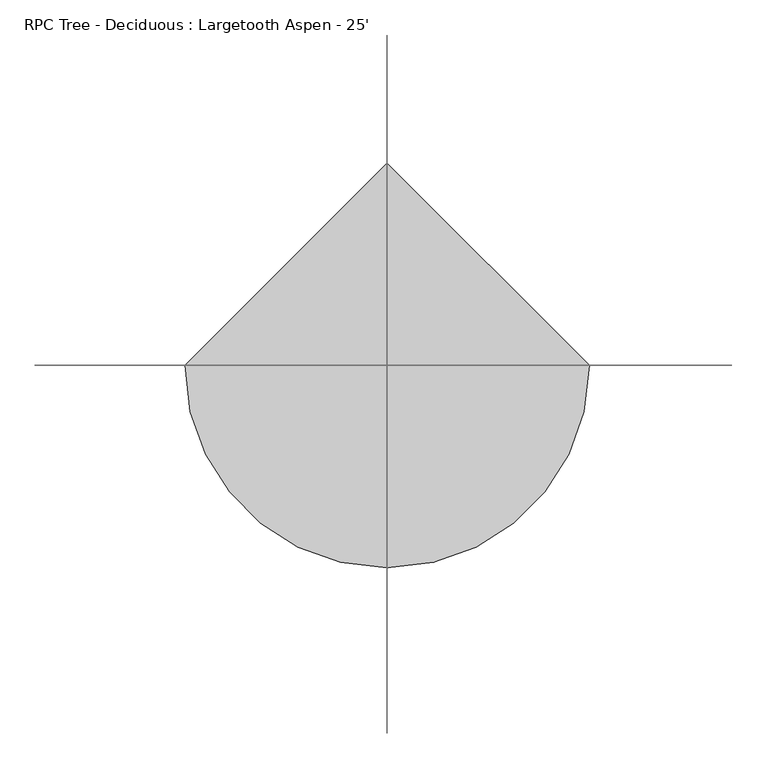
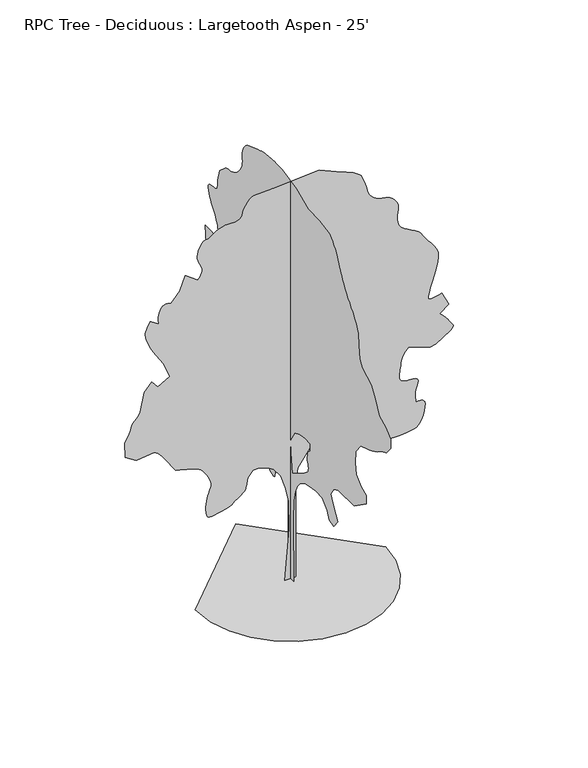
"""IFC4 building model written with IfcOpenShell, lengths in millimetres: geographic element geometry, RPC Tree - Deciduous : Largetooth Aspen - 25'."""

from ifc_helpers import new_model, si_unit, origin, place, context, project, spatial, triangles, source, transform, mapped, element, save


def rpc_tree_deciduous_largetooth_aspen_25_f6cd7aa4(model_context):
    return source(origin(), model_context, "Body", "Tessellation", [
        triangles([(93.1061447, 0.000407, 0.0055275), (-104.1894253, 0.000407, 0.0055275), (-22.9504001, 0.0003503, 951.6658939), (-34.5559031, 0.0003185, 1485.5251682), (-92.5836657, 0.0003019, 1764.061219), (-173.8237105, 0.0002874, 2007.7790462), (-301.4849952, 0.000277, 2181.8628971), (-405.9347789, 0.0002735, 2239.8916225), (-568.4133425, 0.0002701, 2297.9204933), (-684.470866, 0.0002701, 2297.9204933), (-765.710166, 0.000277, 2181.8628971), (-800.5284622, 0.000286, 2030.9895481), (-803.4037228, 0.000287, 2013.4305908), (-808.6158319, 0.0002881, 1994.9546837), (-818.4938627, 0.0002893, 1974.6550507), (-835.3797506, 0.0002907, 1951.6121258), (-861.6001705, 0.0002923, 1924.9168076), (-899.4969126, 0.0002942, 1893.6518555), (-951.4017385, 0.0002963, 1856.9058426), (-1000.9367964, 0.0002984, 1821.7851665), (-1035.041328, 0.0003, 1794.7824543), (-1061.0280413, 0.0003013, 1774.0764507), (-1086.2019407, 0.0003023, 1757.8357269), (-1117.8706472, 0.0003031, 1744.2340862), (-1163.3467958, 0.0003038, 1731.4425705), (-1229.9353912, 0.0003046, 1717.6377445), (-1303.2575146, 0.0003056, 1701.9735844), (-1364.6008633, 0.0003064, 1687.5234489), (-1414.7786144, 0.000307, 1678.356712), (-1454.6032185, 0.000307, 1678.5242889), (-1484.8875618, 0.0003062, 1692.0929375), (-1506.439444, 0.0003043, 1723.119096), (-1520.076693, 0.0003012, 1775.66647), (-1526.0305447, 0.0002975, 1838.229221), (-1525.0830734, 0.000294, 1896.7304466), (-1518.8575813, 0.0002907, 1951.3759483), (-1508.9769344, 0.0002877, 2002.3662952), (-1497.0669056, 0.0002848, 2049.9049633), (-1484.7505062, 0.0002822, 2094.1948471), (-1473.6532185, 0.0002797, 2135.4418934), (-1462.0149754, 0.0002776, 2171.5098953), (-1448.7511047, 0.0002758, 2202.2997311), (-1436.5031605, 0.000274, 2231.0600395), (-1427.9079002, 0.0002723, 2261.0397503), (-1425.6065872, 0.0002702, 2295.4845955), (-1432.2385952, 0.0002677, 2337.6435047), (-1450.4427166, 0.0002645, 2390.7649715), (-1477.2752357, 0.0002611, 2448.2171333), (-1507.353923, 0.000258, 2500.7976448), (-1539.6676483, 0.0002552, 2547.8968048), (-1573.1981598, 0.0002527, 2588.9178474), (-1606.9320019, 0.0002507, 2623.2079056), (-1639.8528122, 0.0002491, 2650.2080017), (-1670.950042, 0.0002479, 2669.3088707), (-1706.2051575, 0.000247, 2684.2184258), (-1751.2088058, 0.0002461, 2699.1535606), (-1804.330418, 0.0002453, 2714.0634064), (-1863.9491627, 0.0002444, 2728.9985413), (-1928.439703, 0.0002435, 2743.908387), (-1996.1788822, 0.0002426, 2758.8182327), (-2065.5412182, 0.0002417, 2773.7533676), (-2262.8354256, 0.0002244, 3063.8972855), (-2307.8392193, 0.0002208, 3124.7302002), (-2344.3134464, 0.0002181, 3169.7390808), (-2373.6809853, 0.0002162, 3201.539756), (-2397.3664581, 0.0002149, 3222.7742157), (-2416.7872204, 0.0002141, 3236.1091576), (-2433.3683304, 0.0002137, 3244.1609917), (-2448.5269981, 0.0002133, 3249.5711266), (-2773.4740242, 0.0002154, 3214.7732506), (-2970.7811668, 0.0002078, 3342.4334816), (-2982.3888885, 0.0001919, 3609.3616653), (-2960.1129227, 0.0001895, 3649.1127274), (-2938.5738304, 0.0001872, 3688.6606041), (-2918.4317459, 0.0001848, 3727.8273994), (-2900.4229614, 0.0001825, 3766.3590591), (-2885.2846413, 0.0001803, 3804.0779778), (-2873.6769196, 0.0001781, 3840.78097), (-2866.3363792, 0.000176, 3876.2901398), (-2854.8809738, 0.000174, 3909.843615), (-2833.1131165, 0.0001721, 3941.5934212), (-2804.8174599, 0.0001702, 3972.5051971), (-2773.8803947, 0.0001684, 4003.6457382), (-2744.1877304, 0.0001665, 4035.9798111), (-2719.5499901, 0.0001644, 4070.5745018), (-2703.8526924, 0.0001621, 4108.3951584), (-2634.2060715, 0.0001414, 4456.5779755), (-2494.950618, 0.0001324, 4607.4283607), (-2390.4982727, 0.00014, 4479.7681297), (-2169.9909473, 0.0001331, 4595.8459282), (-2286.0485435, 0.0001158, 4885.9645569), (-2471.7375, 9.85e-05, 5176.1084747), (-2494.0692764, 9.6e-05, 5217.3577011), (-2519.6494011, 9.3e-05, 5268.7673538), (-2546.0425575, 8.96e-05, 5326.2475662), (-2570.8076157, 8.6e-05, 5385.7596313), (-2591.5086777, 8.26e-05, 5443.2398438), (-2605.7325188, 7.95e-05, 5494.6494965), (-2611.0159172, 7.71e-05, 5535.8993042), (-2608.2980598, 7.5e-05, 5570.3669678), (-2600.7287544, 7.3e-05, 5604.2503647), (-2589.0701637, 7.1e-05, 5637.6006546), (-2574.1858978, 6.9e-05, 5670.544574), (-2556.863118, 6.71e-05, 5703.2088593), (-2537.9197975, 6.52e-05, 5735.6446701), (-2518.1611198, 6.32e-05, 5768.0037415), (-2367.2877708, 6.95e-05, 5663.5595352), (-2372.0934368, 6.75e-05, 5695.9697662), (-2375.8831764, 6.56e-05, 5728.8881058), (-2377.6407726, 6.35e-05, 5762.8226624), (-2376.3555313, 6.14e-05, 5798.2809631), (-2371.00891, 5.92e-05, 5835.7711166), (-2360.5873077, 5.68e-05, 5875.8018127), (-2344.077269, 5.42e-05, 5918.8799973), (-2322.4899239, 5.2e-05, 5956.5480469), (-2297.8569798, 5.05e-05, 5981.4145523), (-2270.6865452, 4.97e-05, 5995.6131042), (-2241.4867287, 4.93e-05, 6001.3028732), (-2210.7630226, 4.94e-05, 6000.5918701), (-2179.0257156, 4.97e-05, 5995.6131042), (-2146.7804455, 5.01e-05, 5988.501329), (-1995.9070965, 3.97e-05, 6162.5924469), (-1891.4573673, 2.45e-05, 6417.9129089), (-1670.950042, 3.42e-05, 6255.4298035), (-1648.8215961, 3.24e-05, 6285.3250717), (-1628.2145691, 3.06e-05, 6315.3988174), (-1610.6529957, 2.88e-05, 6345.8789337), (-1597.6609108, 2.69e-05, 6376.9683151), (-1590.7597332, 2.5e-05, 6408.8960175), (-1591.4684109, 2.31e-05, 6441.814357), (-1601.3160656, 2.1e-05, 6475.9523895), (-1617.3536041, 1.89e-05, 6510.877002), (-1634.407069, 1.68e-05, 6546.3864624), (-1650.6477928, 1.46e-05, 6583.140033), (-1664.2495789, 1.23e-05, 6621.7225616), (-1673.3859398, 9.9e-06, 6662.7183151), (-1676.2282082, 7.3e-06, 6706.761557), (-1670.950042, 4.4e-06, 6754.488295), (-1658.2957272, 1.5e-06, 6803.2306686), (-1640.7672913, -1.2e-06, 6848.9505524), (-1619.1798008, -3.6e-06, 6889.9968842), (-1594.3462875, -5.7e-06, 6924.7441818), (-1567.0742603, -7.3e-06, 6951.5663818), (-1538.1767509, -8.4e-06, 6968.8641632), (-1508.471442, -8.7e-06, 6974.9853012), (-1475.2102455, -9.2e-06, 6983.3417679), (-1435.6574272, -1.05e-05, 7004.9067307), (-1390.6206413, -1.23e-05, 7034.3706299), (-1340.9153904, -1.42e-05, 7066.4762283), (-1287.3545609, -1.59e-05, 7095.9401276), (-1230.7481323, -1.72e-05, 7117.504509), (-1171.9065931, -1.77e-05, 7125.861557), (-1111.9499331, -1.77e-05, 7125.5313446), (-1053.2124573, -1.77e-05, 7125.9882935), (-998.3307781, -1.79e-05, 7129.5188919), (-949.9463768, -1.85e-05, 7138.307309), (-910.695793, -1.94e-05, 7154.6138718), (-883.2205805, -2.1e-05, 7180.6744904), (-870.1599678, -2.32e-05, 7218.6983322), (-859.1973375, -2.62e-05, 7267.6691803), (-837.8816328, -2.94e-05, 7321.8984283), (-808.6488241, -3.27e-05, 7376.76194), (-773.9321205, -3.57e-05, 7427.5367477), (-736.1725794, -3.82e-05, 7469.5992966), (-697.8033371, -3.99e-05, 7498.2504547), (-661.2603642, -4.05e-05, 7508.8422501), (-324.6980224, -4.19e-05, 7532.0576935), (510.9103117, -4.54e-05, 7590.0965927), (928.7119898, -3.43e-05, 7404.3974625), (997.9725878, -3.27e-05, 7376.9148376), (1065.003162, -3.1e-05, 7348.7462082), (1127.5632969, -2.92e-05, 7319.1294113), (1183.4279829, -2.73e-05, 7287.4051849), (1230.3570225, -2.53e-05, 7252.8102036), (1266.1201012, -2.3e-05, 7214.6852051), (1288.4873405, -2.05e-05, 7172.2924438), (1303.3743679, -1.8e-05, 7130.6618454), (1318.0580647, -1.58e-05, 7093.7303787), (1332.3378616, -1.37e-05, 7059.0086609), (1346.0081028, -1.16e-05, 7024.0834671), (1358.8656029, -9.4e-06, 6986.5171555), (1370.7070312, -6.9e-06, 6943.8959198), (1381.3319641, -3.9e-06, 6893.7565384), (1397.2017803, -8e-07, 6841.9149353), (1423.0183731, 2e-06, 6795.9665771), (1455.9391834, 4.3e-06, 6756.1137772), (1493.1248497, 6.3e-06, 6722.5350128), (1531.7301968, 7.9e-06, 6695.4843384), (1568.915863, 9.2e-06, 6675.1134888), (1601.8392895, 1e-05, 6661.6259399), (1632.2912098, 1.04e-05, 6653.548526), (1663.5535458, 1.08e-05, 6648.1133926), (1695.0215378, 1.1e-05, 6643.6683151), (1726.0831593, 1.13e-05, 6638.6389709), (1756.1288544, 1.18e-05, 6631.3492996), (1784.5513927, 1.24e-05, 6620.2238159), (1810.7387478, 1.34e-05, 6603.6126205), (1836.0828403, 1.48e-05, 6581.0320221), (1861.4244621, 1.64e-05, 6553.8028702), (1885.3461124, 1.82e-05, 6522.9169647), (1906.4256397, 2.02e-05, 6489.3887787), (1923.2429272, 2.23e-05, 6454.2351105), (1934.3756779, 2.45e-05, 6418.4721771), (1938.4015949, 2.66e-05, 6383.0900345), (1934.8836411, 2.9e-05, 6341.7640686), (1927.3043072, 3.21e-05, 6289.6434128), (1920.1313438, 3.57e-05, 6230.2325043), (1917.8301762, 3.94e-05, 6166.9613663), (1924.8685547, 4.32e-05, 6103.2838577), (1945.7117592, 4.69e-05, 6042.6538376), (1984.8250694, 5.01e-05, 5988.501329), (2039.569693, 5.28e-05, 5943.162236), (2101.6243355, 5.51e-05, 5904.3256531), (2166.9277622, 5.72e-05, 5868.5371399), (2231.4183025, 5.94e-05, 5832.3166763), (2291.0370472, 6.18e-05, 5792.2609818), (2341.7227615, 6.46e-05, 5744.890036), (2379.4162457, 6.81e-05, 5686.7749786), (2417.9887459, 7.19e-05, 5621.9795151), (2469.1466698, 7.58e-05, 5556.3713104), (2525.585376, 7.98e-05, 5489.1376236), (2580.0024033, 8.4e-05, 5419.4657135), (2625.0618622, 8.83e-05, 5346.5422577), (2653.4845459, 9.29e-05, 5269.5800949), (2657.9549126, 9.78e-05, 5187.7164871), (2641.5719009, 0.0001035, 5093.1519104), (2615.0543335, 0.00011, 4983.9574127), (2582.4409172, 0.0001169, 4868.2862755), (2547.7697777, 0.0001237, 4754.2147499), (2515.1639191, 0.0001299, 4649.8972801), (2488.6361778, 0.000135, 4563.4609863), (2472.2607239, 0.0001386, 4502.9835732), (2471.4479828, 0.0001408, 4466.6872421), (2487.0816216, 0.000142, 4445.6050987), (2516.4161682, 0.0001425, 4437.2230522), (2556.710511, 0.0001424, 4438.9758522), (2605.2247009, 0.0001419, 4448.3482452), (2659.2248932, 0.000141, 4462.8008514), (2715.9685226, 0.00014, 4479.7681297), (2843.6287537, 0.0001552, 4224.4476677), (2681.1706467, 0.0001628, 4096.7874367), (2705.9862831, 0.0001642, 4074.3338654), (2730.6243141, 0.0001655, 4051.3466057), (2754.8559746, 0.000167, 4027.3692902), (2778.4777885, 0.0001685, 4001.8420692), (2801.2868614, 0.0001701, 3974.3085754), (2823.0802986, 0.0001719, 3944.2351204), (2843.6287537, 0.0001739, 3911.1135956), (2865.6250854, 0.0001758, 3878.8553902), (2888.8408195, 0.0001775, 3850.6614716), (2908.8050079, 0.000179, 3824.931356), (2921.0478653, 0.0001805, 3799.9886925), (2921.1240234, 0.0001821, 3774.2329971), (2904.5378265, 0.0001837, 3746.0643677), (2866.8441971, 0.0001857, 3713.8064529), (2611.523735, 0.000196, 3539.7150444), (2507.076622, 0.0001967, 3528.1073227), (2124.0931675, 0.0001891, 3655.7675537), (2096.88727, 0.0001908, 3628.2340599), (2070.5983223, 0.0001925, 3599.5829018), (2046.1355713, 0.0001943, 3568.6964149), (2024.4110252, 0.0001964, 3534.4319366), (2006.3439594, 0.0001987, 3495.74767), (1992.8439114, 0.0002013, 3451.4500832), (1984.8250694, 0.0002043, 3400.4470917), (1979.2422707, 0.0002073, 3350.9425552), (1972.8464401, 0.0002097, 3309.9723816), (1966.2475697, 0.0002118, 3274.6916862), (1960.0550697, 0.0002138, 3242.2305862), (1954.8784962, 0.0002157, 3209.7947754), (1951.3250793, 0.0002178, 3174.4887909), (1950.0068459, 0.0002203, 3133.5186172), (1959.0060059, 0.0002226, 3094.8599304), (1982.2191238, 0.0002242, 3067.1485405), (2013.9564308, 0.0002253, 3048.55578), (2048.5358608, 0.000226, 3037.3035599), (2080.2731678, 0.0002263, 3031.5123436), (2103.4861404, 0.0002265, 3029.3787529), (2112.4854458, 0.0002265, 3029.0738297), (2125.1752235, 0.0002264, 3029.9630196), (2157.148708, 0.0002264, 3030.4202591), (2199.274625, 0.0002266, 3027.2451622), (2242.4164684, 0.0002272, 3017.1614754), (2277.4354065, 0.0002284, 2996.942942), (2295.2001652, 0.0002304, 2963.2880196), (2286.5717674, 0.0002334, 2913.021611), (2265.7615551, 0.0002368, 2855.3635025), (2252.261507, 0.0002401, 2801.3633102), (2244.8497501, 0.0002431, 2750.4108971), (2242.3122597, 0.000246, 2701.871418), (2243.429924, 0.0002488, 2655.1864769), (2246.9833408, 0.0002515, 2609.7203568), (2251.7533985, 0.0002541, 2564.8385033), (2291.2047695, 0.0002539, 2569.2835808), (2328.629084, 0.0002538, 2570.4774033), (2361.9894024, 0.0002541, 2565.1434265), (2389.2612843, 0.000255, 2550.1065536), (2408.4128769, 0.0002567, 2522.0472198), (2417.4120369, 0.0002593, 2477.7574814), (2414.2319984, 0.0002631, 2413.9754734), (2401.476091, 0.0002675, 2341.0953289), (2383.2389774, 0.0002716, 2272.8811787), (2359.7236977, 0.0002752, 2211.166777), (2331.1309662, 0.0002784, 2157.7735245), (2297.6690552, 0.000281, 2114.5300884), (2259.536063, 0.0002829, 2083.2677525), (2216.9377911, 0.0002839, 2065.807917), (2176.9759861, 0.0002844, 2057.1795193), (2143.1075592, 0.0002848, 2050.7838341), (2110.049548, 0.0002851, 2046.0136311), (2072.5261116, 0.0002853, 2042.257029), (2025.2567585, 0.0002855, 2038.9092682), (1962.9659386, 0.0002857, 2035.3558514), (1880.3728695, 0.000286, 2030.9895481), (1790.6068371, 0.0002859, 2032.4449825), (1709.3674644, 0.0002851, 2045.4726757), (1635.2326, 0.0002838, 2068.1420769), (1566.7847431, 0.0002819, 2098.5255421), (1502.5989807, 0.0002798, 2134.6977528), (1441.2554867, 0.0002774, 2174.7255421), (1381.3319641, 0.0002749, 2216.6811207), (1126.0062698, 0.0002604, 2460.3989479), (859.0779408, 0.0002535, 2576.4465157), (545.7260645, 0.0002548, 2553.2563614), (394.8527518, 0.0002618, 2437.1885914), (290.4029863, 0.0002708, 2286.3152424), (127.9229058, 0.0002846, 2054.2026661), (93.1061447, 0.0003019, 1764.061219), (93.1061447, 0.0003392, 1137.3575392), (-0.0023708, 90.8437737, 1.11e-05), (-0.0023708, -94.8460457, 0.0), (-0.0023708, -83.2405405, 1160.5629541), (-0.0023708, -94.8460457, 1531.9435558), (-0.0023708, -141.2688208, 1729.2379086), (-0.0023708, -210.9025882, 1880.1112576), (-0.0023708, -303.7481383, 1996.1687084), (-0.0023708, -443.0162001, 2077.4080811), (-0.0023708, -559.0712165, 2100.6185829), (-0.0023708, -791.1838291, 2147.0420574), (-0.0023708, -988.4806526, 2135.4368065), (-0.0023708, -1139.3539289, 1984.5634575), (-0.0023708, -1208.987978, 1845.2955048), (-0.0023708, -1336.648209, 1798.8718849), (-0.0023708, -1475.9163071, 1972.9557358), (-0.0023708, -1325.0429581, 2205.0707829), (-0.0023708, -1255.4089817, 2367.5493828), (-0.0023708, -1336.648209, 2506.8150101), (-0.0023708, -1487.521558, 2576.4465157), (-0.0023708, -1974.9572124, 2576.4465157), (-0.0023708, -2357.9431377, 2843.3746994), (-0.0023708, -2357.9431377, 3005.8583862), (-0.0023708, -2195.4645378, 3075.479718), (-0.0023708, -2044.5913342, 3214.7476707), (-0.0023708, -2009.7755814, 3412.0548134), (-0.0023708, -2032.9860832, 3644.159832), (-0.0023708, -2183.8592869, 3841.466684), (-0.0023708, -2450.787616, 3934.3037498), (-0.0023708, -2495.4866318, 3951.778846), (-0.0023708, -2539.7763702, 3969.5332855), (-0.0023708, -2583.2536583, 3987.8975716), (-0.0023708, -2625.5191017, 4007.2016258), (-0.0023708, -2666.159063, 4027.6995026), (-0.0023708, -2704.7671715, 4049.7211235), (-0.0023708, -2740.9367661, 4073.5717026), (-0.0023708, -2775.734642, 4097.0920692), (-0.0023708, -2810.5580978, 4118.1742126), (-0.0023708, -2845.381263, 4137.223922), (-0.0023708, -2880.2047188, 4154.6484398), (-0.0023708, -2915.0025948, 4170.8535553), (-0.0023708, -2949.8260506, 4186.2459297), (-0.0023708, -2984.6495064, 4201.2319336), (-0.0023708, -3112.3097374, 4363.7156204), (-0.0023708, -3112.3097374, 4526.1993073), (-0.0023708, -2961.4337723, 4665.46726), (-0.0023708, -2764.1522095, 4769.9120476), (-0.0023708, -2636.4666893, 5013.6247879), (-0.0023708, -2508.8189575, 5199.3239182), (-0.0023708, -2230.2829067, 5350.1995926), (-0.0023708, -2149.0435341, 5477.860405), (-0.0023708, -2125.8305614, 5733.180867), (-0.0023708, -2102.6200596, 5942.0698608), (-0.0023708, -2077.7179459, 5994.1655182), (-0.0023708, -2052.6126469, 6045.3211166), (-0.0023708, -2027.0983612, 6094.647757), (-0.0023708, -2000.9769905, 6141.2315414), (-0.0023708, -1974.0453495, 6184.1824081), (-0.0023708, -1946.0953114, 6222.5364624), (-0.0023708, -1916.9309578, 6255.4298035), (-0.0023708, -1880.7588924, 6294.3169647), (-0.0023708, -1835.0490372, 6347.6061539), (-0.0023708, -1784.4624447, 6409.8360764), (-0.0023708, -1733.6777538, 6475.4948593), (-0.0023708, -1687.355872, 6539.1473694), (-0.0023708, -1650.170351, 6595.2811523), (-0.0023708, -1626.7896561, 6638.4104965), (-0.0023708, -1609.9062389, 6674.6559586), (-0.0023708, -1589.7741829, 6713.7465958), (-0.0023708, -1567.4070889, 6755.6568283), (-0.0023708, -1543.8256794, 6800.4366531), (-0.0023708, -1520.0386139, 6848.0360733), (-0.0023708, -1497.0642895, 6898.4806686), (-0.0023708, -1475.9163071, 6951.7698578), (-0.0023708, -1452.6372047, 7005.1352051), (-0.0023708, -1423.2671951, 7056.0623291), (-0.0023708, -1388.8223499, 7104.957019), (-0.0023708, -1350.3185955, 7152.2262268), (-0.0023708, -1308.7667713, 7198.2763229), (-0.0023708, -1265.188036, 7243.513678), (-0.0023708, -1220.5932289, 7288.3446625), (-0.0023708, -895.6335583, 7346.3585632), (-0.0023708, -547.4659656, 7357.9659943), (-0.0023708, -176.0855819, 7520.4496811), (-0.0023708, 264.9268161, 7613.2870377), (-0.0023708, 324.5456334, 7615.7252609), (-0.0023708, 383.7580439, 7617.8588516), (-0.0023708, 442.1602203, 7619.3825958), (-0.0023708, 499.3406327, 7619.9924423), (-0.0023708, 554.9005408, 7619.3825958), (-0.0023708, 608.4284509, 7617.2490051), (-0.0023708, 659.5204994, 7613.2870377), (-0.0023708, 708.649114, 7608.2065338), (-0.0023708, 756.9649876, 7602.5423447), (-0.0023708, 805.0801466, 7595.6340454), (-0.0023708, 853.6016762, 7586.8962067), (-0.0023708, 903.136734, 7575.7457245), (-0.0023708, 954.2948032, 7561.5215927), (-0.0023708, 1007.6881285, 7543.6657059), (-0.0023708, 1344.2529774, 7427.6129059), (-0.0023708, 1373.9607571, 7402.5429245), (-0.0023708, 1402.8557957, 7376.228833), (-0.0023708, 1430.1278229, 7347.5015167), (-0.0023708, 1454.9613361, 7315.141864), (-0.0023708, 1476.5488266, 7277.8801849), (-0.0023708, 1494.0772625, 7234.5479462), (-0.0023708, 1506.7315773, 7183.8748764), (-0.0023708, 1511.0952644, 7135.4627151), (-0.0023708, 1507.5418476, 7096.3970764), (-0.0023708, 1500.9454479, 7061.7770966), (-0.0023708, 1496.1727741, 7026.7507462), (-0.0023708, 1498.1031796, 6986.4659958), (-0.0023708, 1511.6032276, 6935.996402), (-0.0023708, 1541.5473301, 6870.5405136), (-0.0023708, 1582.5555828, 6804.0434097), (-0.0023708, 1625.189463, 6752.1768082), (-0.0023708, 1668.2270977, 6712.4769058), (-0.0023708, 1710.4546074, 6682.5298965), (-0.0023708, 1750.6525898, 6659.8987198), (-0.0023708, 1787.5994625, 6642.1439896), (-0.0023708, 1820.0833809, 6626.8024841), (-0.0023708, 1849.9258907, 6615.6775818), (-0.0023708, 1879.7682552, 6610.2418671), (-0.0023708, 1909.6107651, 6607.6257477), (-0.0023708, 1939.4557457, 6605.0346268), (-0.0023708, 1969.2981102, 6599.5739136), (-0.0023708, 1999.14062, 6588.4484299), (-0.0023708, 2028.9829845, 6568.7891647), (-0.0023708, 2203.0693062, 6417.9129089), (-0.0023708, 2272.7008118, 6197.4159027), (-0.0023708, 2270.435107, 6162.7197647), (-0.0023708, 2269.4877811, 6128.8613663), (-0.0023708, 2271.179393, 6096.6034515), (-0.0023708, 2276.8307922, 6066.8093399), (-0.0023708, 2287.7578869, 6040.2411942), (-0.0023708, 2305.2864681, 6017.7367538), (-0.0023708, 2330.7295372, 6000.1087601), (-0.0023708, 2366.121999, 5990.0250732), (-0.0023708, 2409.2282341, 5986.2404205), (-0.0023708, 2454.9736977, 5983.6754608), (-0.0023708, 2498.2855888, 5977.2491089), (-0.0023708, 2534.0819504, 5961.8820236), (-0.0023708, 2557.2947777, 5932.4942825), (-0.0023708, 2562.8319397, 5884.0565414), (-0.0023708, 2554.1452606, 5827.7448624), (-0.0023708, 2538.7528862, 5777.5287415), (-0.0023708, 2517.7724808, 5732.3931244), (-0.0023708, 2492.3292664, 5691.3217941), (-0.0023708, 2463.5359657, 5653.2979523), (-0.0023708, 2432.5073364, 5617.3059631), (-0.0023708, 2400.3636589, 5582.3046112), (-0.0023708, 2375.59613, 5540.0391678), (-0.0023708, 2351.4381569, 5497.9004608), (-0.0023708, 2328.49697, 5455.9402313), (-0.0023708, 2307.3844505, 5414.284053), (-0.0023708, 2288.7053581, 5373.0342453), (-0.0023708, 2273.0741901, 5332.2931274), (-0.0023708, 2261.0955608, 5292.1606934), (-0.0023708, 2254.8700687, 5254.4164856), (-0.0023708, 2255.3450397, 5220.3046143), (-0.0023708, 2261.4003387, 5189.2402313), (-0.0023708, 2271.9235336, 5160.614653), (-0.0023708, 2285.7971054, 5133.8174515), (-0.0023708, 2301.9032444, 5108.2399429), (-0.0023708, 2319.1244316, 5083.2716995), (-0.0023708, 2469.9977806, 5106.4871429), (-0.0023708, 2655.6942947, 5106.4871429), (-0.0023708, 2632.4788513, 4769.9120476), (-0.0023708, 2423.5741608, 4410.1467979), (-0.0023708, 2416.0988903, 4367.9066437), (-0.0023708, 2408.5195564, 4325.9967018), (-0.0023708, 2400.7370373, 4284.6710266), (-0.0023708, 2392.6495949, 4244.2848289), (-0.0023708, 2384.1559273, 4205.0927444), (-0.0023708, 2375.1567673, 4167.4246948), (-0.0023708, 2365.5479061, 4131.6106018), (-0.0023708, 2351.1663712, 4092.901046), (-0.0023708, 2330.0869892, 4047.8924561), (-0.0023708, 2305.5556377, 3998.8448685), (-0.0023708, 2280.8237171, 3947.9433243), (-0.0023708, 2259.134634, 3897.4737305), (-0.0023708, 2243.7397888, 3849.620256), (-0.0023708, 2237.885059, 3806.6435188), (-0.0023708, 2242.6221245, 3768.5435188), (-0.0023708, 2255.8859951, 3733.4915886), (-0.0023708, 2276.2542286, 3700.9796196), (-0.0023708, 2302.3069988, 3670.4995033), (-0.0023708, 2332.6244797, 3641.5181328), (-0.0023708, 2365.7840836, 3613.5782684), (-0.0023708, 2400.3636589, 3586.1462219), (-0.0023708, 2713.7079048, 3655.7675537), (-0.0023708, 2731.0053955, 3606.110701), (-0.0023708, 2747.5915924, 3556.834639), (-0.0023708, 2762.7552017, 3508.3968979), (-0.0023708, 2775.7599312, 3461.1529793), (-0.0023708, 2785.945356, 3415.5345428), (-0.0023708, 2792.5748932, 3371.9482498), (-0.0023708, 2794.9625381, 3330.8257599), (-0.0023708, 2781.5002785, 3291.6333847), (-0.0023708, 2746.9055878, 3253.2540413), (-0.0023708, 2699.9410126, 3215.103463), (-0.0023708, 2649.3188118, 3176.5209343), (-0.0023708, 2603.7768242, 3136.9477684), (-0.0023708, 2572.0523071, 3095.7235405), (-0.0023708, 2562.8319397, 3052.2895638), (-0.0023708, 2571.1886971, 3010.557518), (-0.0023708, 2585.6413033, 2974.3117653), (-0.0023708, 2605.1738319, 2942.6631157), (-0.0023708, 2628.7450676, 2914.6470932), (-0.0023708, 2655.3896622, 2889.3742172), (-0.0023708, 2684.0408203, 2865.9044289), (-0.0023708, 2713.7079048, 2843.3746994), (-0.0023708, 2783.3545258, 2611.2696808), (-0.0023708, 2716.5272095, 2608.9584846), (-0.0023708, 2651.6302986, 2607.7899513), (-0.0023708, 2590.5941986, 2608.8314575), (-0.0023708, 2535.3339088, 2613.225666), (-0.0023708, 2487.7955315, 2622.0902412), (-0.0023708, 2449.8987167, 2636.5428474), (-0.0023708, 2423.5741608, 2657.7008583), (-0.0023708, 2398.2655312, 2683.9137932), (-0.0023708, 2363.2136009, 2712.5649513), (-0.0023708, 2320.0387653, 2743.2479622), (-0.0023708, 2270.3665066, 2775.5823257), (-0.0023708, 2215.8225975, 2809.1102211), (-0.0023708, 2158.0326656, 2843.4508575), (-0.0023708, 2098.6169609, 2878.1981552), (-0.0023708, 2096.1482162, 2840.8347382), (-0.0023708, 2093.7783028, 2803.1919777), (-0.0023708, 2091.6141907, 2764.9143723), (-0.0023708, 2089.7523857, 2725.7219971), (-0.0023708, 2088.2969513, 2685.3360901), (-0.0023708, 2087.3496254, 2643.4008591), (-0.0023708, 2087.01171, 2599.6619591), (-0.0023708, 2085.4216908, 2554.0943916), (-0.0023708, 2079.9734768, 2509.3195084), (-0.0023708, 2069.6534672, 2469.0222588), (-0.0023708, 2053.4457355, 2436.8431183), (-0.0023708, 2030.3368263, 2416.4418926), (-0.0023708, 1999.3108131, 2411.4660336), (-0.0023708, 1959.3490082, 2425.5756374), (-0.0023708, 1914.2462379, 2451.7986008), (-0.0023708, 1868.5363827, 2480.4573166), (-0.0023708, 1822.3160934, 2511.1455597), (-0.0023708, 1775.6894337, 2543.4517273), (-0.0023708, 1728.7603214, 2576.9799133), (-0.0023708, 1681.6281693, 2611.3461296), (-0.0023708, 1634.3918083, 2646.0931366), (-0.0023708, 1355.8582283, 2727.3221901), (-0.0023708, 1077.3221775, 2634.4854149), (-0.0023708, 903.2383266, 2425.5756374), (-0.0023708, 925.671623, 2395.8678577), (-0.0023708, 948.4096247, 2366.9728191), (-0.0023708, 971.754784, 2339.7009373), (-0.0023708, 996.0142771, 2314.8672787), (-0.0023708, 1021.4930271, 2293.2799335), (-0.0023708, 1048.4931959, 2275.7513523), (-0.0023708, 1077.3221775, 2263.0970375), (-0.0023708, 1104.7973173, 2250.7806381), (-0.0023708, 1128.0078192, 2234.2021442), (-0.0023708, 1147.667375, 2214.0700882), (-0.0023708, 1164.4821917, 2191.0957638), (-0.0023708, 1179.1684319, 2165.9904648), (-0.0023708, 1192.4323025, 2139.4627235), (-0.0023708, 1204.984952, 2112.2238338), (-0.0023708, 1172.5694887, 2104.7129551), (-0.0023708, 1139.6486057, 2096.8974438), (-0.0023708, 1105.7091803, 2088.4722313), (-0.0023708, 1070.2508068, 2079.1326851), (-0.0023708, 1032.7604353, 2068.576498), (-0.0023708, 992.7325733, 2056.4962761), (-0.0023708, 949.6593304, 2042.5897121), (-0.0023708, 906.5885582, 2025.6403107), (-0.0023708, 866.5607689, 2005.0332836), (-0.0023708, 829.0703974, 1981.383419), (-0.0023708, 793.6094805, 1955.2951859), (-0.0023708, 759.6725985, 1927.3806107), (-0.0023708, 726.7517155, 1898.2467785), (-0.0023708, 694.3362522, 1868.5060066), (-0.0023708, 694.3362522, 1706.0274067), (-0.0023708, 652.3120005, 1679.1287579), (-0.0023708, 611.8117109, 1654.968314), (-0.0023708, 574.3543679, 1636.2916924), (-0.0023708, 541.4665134, 1625.8370979), (-0.0023708, 514.6695299, 1626.3450611), (-0.0023708, 495.4849088, 1640.556403), (-0.0023708, 485.4341414, 1671.2116539), (-0.0023708, 480.5294263, 1705.9588062), (-0.0023708, 476.0285382, 1733.1976959), (-0.0023708, 472.3404639, 1756.7815762), (-0.0023708, 469.8715739, 1780.5661709), (-0.0023708, 469.025768, 1808.4147617), (-0.0023708, 470.2094167, 1844.1778404), (-0.0023708, 473.8288905, 1891.7165085), (-0.0023708, 476.7727515, 1943.7229271), (-0.0023708, 476.0615667, 1990.8550793), (-0.0023708, 472.3074354, 2033.9283222), (-0.0023708, 466.1149355, 2073.7529263), (-0.0023708, 458.0961662, 2111.1417778), (-0.0023708, 448.8581763, 2146.9074726), (-0.0023708, 439.0131741, 2181.8578102), (-0.0023708, 241.7168229, 2193.4630611), (-0.0023708, 137.2665396, 1996.1687084), (-0.0023708, 79.2382684, 1659.6039322), (-0.0023708, 79.2382684, 1230.1970032), (-0.0023708, 79.2382684, 591.8879997), (-0.0022508, -48.4240337, 2030.9844612), (-0.0022508, -2.0012081, 2402.3651356), (-0.0022508, 9.6043397, 2622.8776932), (-0.0022508, -129.6633155, 2843.3746994), (-0.0022508, -280.5376365, 2913.021611), (-0.0022508, -454.621451, 2936.2117653), (-0.0022508, -617.0999783, 2936.2117653), (-0.0022508, -617.0999783, 2796.9691017), (-0.0022508, -535.8607146, 2727.3221901), (-0.0022508, -512.6502128, 2564.8385033), (-0.0022508, -522.5282799, 2554.7295273), (-0.0022508, -532.0024836, 2543.6043343), (-0.0022508, -540.6638735, 2530.4344986), (-0.0022508, -548.1085862, 2514.226767), (-0.0022508, -553.9277441, 2493.9573647), (-0.0022508, -557.717411, 2468.6158882), (-0.0022508, -559.0712165, 2437.1808884), (-0.0022508, -555.6879564, 2404.7324329), (-0.0022508, -546.2137527, 2376.5486881), (-0.0022508, -531.6646408, 2351.915744), (-0.0022508, -513.0540762, 2330.1250683), (-0.0022508, -491.4006014, 2310.4679832), (-0.0022508, -467.7151285, 2292.2308697), (-0.0022508, -443.0162001, 2274.7022884), (-1711.8591728, 0.0, 0.0031267), (-1666.6040863, -392.2441901, 0.0031033), (-1537.7144245, -752.4590126, 0.0030819), (-1335.5154293, -1070.3218781, 0.0030629), (-1070.3218781, -1335.5154293, 0.0030471), (-752.4590126, -1537.7144245, 0.0030351), (-392.2441901, -1666.6040863, 0.0030274), (7.5e-05, -1711.8591728, 0.0030247), (392.2441901, -1666.6040863, 0.0030274), (752.4590126, -1537.7144245, 0.0030351), (1070.3218781, -1335.5154293, 0.0030471), (1335.5154293, -1070.3218781, 0.0030629), (1537.7144245, -752.4590126, 0.0030819), (1666.6040863, -392.2441901, 0.0031033), (1711.8591728, 0.0001497, 0.0031267), (-0.0002251, 1711.8591728, 0.0032287)], [[122, 123, 124], [87, 88, 89], [1, 2, 3], [329, 1, 3], [329, 3, 4], [328, 329, 4], [328, 4, 5], [105, 106, 107], [327, 328, 5], [327, 5, 6], [104, 105, 107], [238, 239, 240], [238, 240, 241], [237, 238, 241], [236, 237, 241], [103, 104, 107], [86, 87, 89], [235, 236, 241], [102, 103, 107], [101, 102, 107], [100, 101, 107], [99, 100, 107], [98, 99, 107], [97, 98, 107], [96, 97, 107], [327, 6, 7], [326, 327, 7], [95, 96, 107], [70, 71, 72], [69, 70, 72], [69, 72, 73], [69, 73, 74], [69, 74, 75], [69, 75, 76], [69, 76, 77], [69, 77, 78], [94, 95, 107], [234, 235, 241], [93, 94, 107], [69, 78, 79], [69, 79, 80], [69, 80, 81], [69, 81, 82], [69, 82, 83], [69, 83, 84], [69, 84, 85], [68, 69, 85], [325, 326, 7], [325, 7, 8], [67, 68, 85], [92, 93, 107], [91, 92, 107], [60, 61, 62], [67, 85, 86], [67, 86, 89], [67, 89, 90], [66, 67, 90], [65, 66, 90], [64, 65, 90], [63, 64, 90], [62, 63, 90], [60, 62, 90], [59, 60, 90], [58, 59, 90], [57, 58, 90], [56, 57, 90], [55, 56, 90], [54, 55, 90], [53, 54, 90], [284, 285, 286], [283, 284, 286], [282, 283, 286], [282, 286, 287], [281, 282, 287], [280, 281, 287], [279, 280, 287], [279, 287, 288], [278, 279, 288], [277, 278, 288], [277, 288, 289], [276, 277, 289], [275, 276, 289], [275, 289, 290], [52, 53, 90], [325, 8, 9], [121, 122, 124], [275, 290, 291], [30, 31, 32], [29, 30, 32], [29, 32, 33], [28, 29, 33], [28, 33, 34], [27, 28, 34], [27, 34, 35], [27, 35, 36], [26, 27, 36], [26, 36, 37], [26, 37, 38], [25, 26, 38], [25, 38, 39], [24, 25, 39], [23, 24, 39], [22, 23, 39], [21, 22, 39], [20, 21, 39], [20, 39, 40], [20, 40, 41], [20, 41, 42], [19, 20, 42], [19, 42, 43], [18, 19, 43], [18, 43, 44], [17, 18, 44], [16, 17, 44], [15, 16, 44], [14, 15, 44], [13, 14, 44], [12, 13, 44], [11, 12, 44], [11, 44, 45], [11, 45, 46], [10, 11, 46], [10, 46, 47], [10, 47, 48], [10, 48, 49], [10, 49, 50], [10, 50, 51], [252, 253, 254], [251, 252, 254], [251, 254, 255], [250, 251, 255], [249, 250, 255], [249, 255, 256], [248, 249, 256], [247, 248, 256], [246, 247, 256], [245, 246, 256], [245, 256, 257], [245, 257, 258], [244, 245, 258], [243, 244, 258], [242, 243, 258], [241, 242, 258], [234, 241, 258], [233, 234, 258], [274, 275, 291], [324, 325, 9], [51, 52, 90], [10, 51, 90], [9, 10, 90], [324, 9, 90], [323, 324, 90], [323, 90, 91], [323, 91, 107], [323, 107, 108], [323, 108, 109], [323, 109, 110], [323, 110, 111], [323, 111, 112], [323, 112, 113], [323, 113, 114], [323, 114, 115], [323, 115, 116], [323, 116, 117], [323, 117, 118], [323, 118, 119], [323, 119, 120], [323, 120, 121], [323, 121, 124], [323, 124, 125], [323, 125, 126], [323, 126, 127], [323, 127, 128], [323, 128, 129], [322, 323, 129], [322, 129, 130], [167, 168, 169], [274, 291, 292], [296, 297, 298], [296, 298, 299], [295, 296, 299], [294, 295, 299], [294, 299, 300], [293, 294, 300], [293, 300, 301], [293, 301, 302], [293, 302, 303], [293, 303, 304], [293, 304, 305], [293, 305, 306], [293, 306, 307], [293, 307, 308], [293, 308, 309], [293, 309, 310], [293, 310, 311], [293, 311, 312], [293, 312, 313], [293, 313, 314], [293, 314, 315], [293, 315, 316], [293, 316, 317], [293, 317, 318], [293, 318, 319], [292, 293, 319], [274, 292, 319], [274, 319, 320], [274, 320, 321], [274, 321, 322], [273, 274, 322], [273, 322, 130], [272, 273, 130], [271, 272, 130], [270, 271, 130], [269, 270, 130], [268, 269, 130], [267, 268, 130], [266, 267, 130], [265, 266, 130], [264, 265, 130], [263, 264, 130], [262, 263, 130], [261, 262, 130], [260, 261, 130], [259, 260, 130], [258, 259, 130], [233, 258, 130], [232, 233, 130], [231, 232, 130], [230, 231, 130], [229, 230, 130], [228, 229, 130], [227, 228, 130], [226, 227, 130], [225, 226, 130], [224, 225, 130], [223, 224, 130], [222, 223, 130], [221, 222, 130], [220, 221, 130], [219, 220, 130], [218, 219, 130], [217, 218, 130], [216, 217, 130], [215, 216, 130], [214, 215, 130], [213, 214, 130], [212, 213, 130], [211, 212, 130], [210, 211, 130], [209, 210, 130], [208, 209, 130], [207, 208, 130], [206, 207, 130], [205, 206, 130], [204, 205, 130], [203, 204, 130], [202, 203, 130], [201, 202, 130], [200, 201, 130], [199, 200, 130], [198, 199, 130], [197, 198, 130], [196, 197, 130], [195, 196, 130], [194, 195, 130], [193, 194, 130], [192, 193, 130], [191, 192, 130], [190, 191, 130], [189, 190, 130], [188, 189, 130], [187, 188, 130], [186, 187, 130], [185, 186, 130], [184, 185, 130], [183, 184, 130], [182, 183, 130], [181, 182, 130], [180, 181, 130], [179, 180, 130], [178, 179, 130], [177, 178, 130], [176, 177, 130], [175, 176, 130], [174, 175, 130], [173, 174, 130], [172, 173, 130], [171, 172, 130], [170, 171, 130], [169, 170, 130], [167, 169, 130], [167, 130, 131], [167, 131, 132], [167, 132, 133], [167, 133, 134], [167, 134, 135], [167, 135, 136], [164, 165, 166], [164, 166, 167], [163, 164, 167], [162, 163, 167], [161, 162, 167], [160, 161, 167], [159, 160, 167], [158, 159, 167], [143, 144, 145], [142, 143, 145], [141, 142, 145], [140, 141, 145], [140, 145, 146], [139, 140, 146], [138, 139, 146], [137, 138, 146], [136, 137, 146], [136, 146, 147], [136, 147, 148], [136, 148, 149], [136, 149, 150], [136, 150, 151], [136, 151, 152], [136, 152, 153], [136, 153, 154], [136, 154, 155], [136, 155, 156], [157, 158, 167], [157, 167, 136], [157, 136, 156], [634, 330, 635], [633, 634, 635], [632, 633, 635], [631, 632, 635], [540, 541, 542], [592, 593, 594], [494, 495, 496], [635, 330, 331], [635, 331, 332], [635, 332, 333], [635, 333, 334], [635, 334, 335], [658, 635, 335], [658, 335, 336], [658, 336, 337], [658, 337, 338], [540, 542, 543], [657, 658, 338], [631, 635, 636], [630, 631, 636], [518, 519, 520], [656, 657, 338], [656, 338, 339], [655, 656, 339], [654, 655, 339], [653, 654, 339], [540, 543, 544], [539, 540, 544], [518, 520, 521], [539, 544, 545], [538, 539, 545], [538, 545, 546], [538, 546, 547], [538, 547, 548], [537, 538, 548], [537, 548, 549], [536, 537, 549], [536, 549, 550], [536, 550, 551], [535, 536, 551], [535, 551, 552], [534, 535, 552], [493, 494, 496], [493, 496, 497], [343, 344, 345], [342, 343, 345], [341, 342, 345], [340, 341, 345], [340, 345, 346], [534, 552, 553], [533, 534, 553], [518, 521, 522], [350, 351, 352], [349, 350, 352], [349, 352, 353], [348, 349, 353], [533, 553, 554], [652, 653, 339], [518, 522, 523], [518, 523, 524], [533, 554, 555], [532, 533, 555], [518, 524, 525], [518, 525, 526], [518, 526, 527], [518, 527, 528], [518, 528, 529], [518, 529, 530], [518, 530, 531], [518, 531, 532], [518, 532, 555], [517, 518, 555], [516, 517, 555], [515, 516, 555], [607, 608, 609], [591, 592, 594], [591, 594, 595], [590, 591, 595], [590, 595, 596], [589, 590, 596], [588, 589, 596], [588, 596, 597], [587, 588, 597], [586, 587, 597], [586, 597, 598], [585, 586, 598], [585, 598, 599], [584, 585, 599], [584, 599, 600], [583, 584, 600], [583, 600, 601], [582, 583, 601], [514, 515, 555], [643, 644, 645], [630, 636, 637], [629, 630, 637], [581, 582, 601], [581, 601, 602], [348, 353, 354], [580, 581, 602], [580, 602, 603], [579, 580, 603], [651, 652, 339], [651, 339, 340], [651, 340, 346], [650, 651, 346], [649, 650, 346], [649, 346, 347], [648, 649, 347], [647, 648, 347], [646, 647, 347], [372, 373, 374], [371, 372, 374], [370, 371, 374], [369, 370, 374], [369, 374, 375], [368, 369, 375], [367, 368, 375], [366, 367, 375], [365, 366, 375], [364, 365, 375], [363, 364, 375], [362, 363, 375], [361, 362, 375], [360, 361, 375], [359, 360, 375], [358, 359, 375], [357, 358, 375], [356, 357, 375], [356, 375, 376], [356, 376, 377], [356, 377, 378], [645, 646, 347], [643, 645, 347], [642, 643, 347], [641, 642, 347], [641, 347, 348], [641, 348, 354], [641, 354, 355], [607, 609, 610], [513, 514, 555], [579, 603, 604], [607, 610, 611], [607, 611, 612], [607, 612, 613], [607, 613, 614], [607, 614, 615], [607, 615, 616], [607, 616, 617], [607, 617, 618], [607, 618, 619], [607, 619, 620], [607, 620, 621], [607, 621, 622], [607, 622, 623], [607, 623, 624], [606, 607, 624], [606, 624, 625], [605, 606, 625], [605, 625, 626], [604, 605, 626], [579, 604, 626], [579, 626, 627], [579, 627, 628], [579, 628, 629], [579, 629, 637], [578, 579, 637], [578, 637, 638], [355, 356, 378], [641, 355, 378], [641, 378, 379], [640, 641, 379], [639, 640, 379], [639, 379, 380], [639, 380, 381], [639, 381, 382], [639, 382, 383], [639, 383, 384], [639, 384, 385], [639, 385, 386], [639, 386, 387], [639, 387, 388], [639, 388, 389], [639, 389, 390], [639, 390, 391], [639, 391, 392], [639, 392, 393], [639, 393, 394], [639, 394, 395], [638, 639, 395], [578, 638, 395], [577, 578, 395], [577, 395, 396], [577, 396, 397], [577, 397, 398], [577, 398, 399], [577, 399, 400], [577, 400, 401], [577, 401, 402], [577, 402, 403], [577, 403, 404], [577, 404, 405], [577, 405, 406], [577, 406, 407], [577, 407, 408], [577, 408, 409], [577, 409, 410], [577, 410, 411], [577, 411, 412], [577, 412, 413], [577, 413, 414], [577, 414, 415], [577, 415, 416], [577, 416, 417], [577, 417, 418], [577, 418, 419], [577, 419, 420], [577, 420, 421], [577, 421, 422], [577, 422, 423], [577, 423, 424], [577, 424, 425], [577, 425, 426], [577, 426, 427], [577, 427, 428], [577, 428, 429], [577, 429, 430], [577, 430, 431], [577, 431, 432], [577, 432, 433], [577, 433, 434], [566, 567, 568], [566, 568, 569], [565, 566, 569], [564, 565, 569], [564, 569, 570], [563, 564, 570], [563, 570, 571], [562, 563, 571], [562, 571, 572], [561, 562, 572], [560, 561, 572], [560, 572, 573], [559, 560, 573], [559, 573, 574], [558, 559, 574], [558, 574, 575], [557, 558, 575], [556, 557, 575], [556, 575, 576], [555, 556, 576], [513, 555, 576], [513, 576, 577], [512, 513, 577], [511, 512, 577], [470, 471, 472], [469, 470, 472], [468, 469, 472], [468, 472, 473], [467, 468, 473], [467, 473, 474], [467, 474, 475], [466, 467, 475], [466, 475, 476], [466, 476, 477], [465, 466, 477], [465, 477, 478], [465, 478, 479], [464, 465, 479], [464, 479, 480], [464, 480, 481], [464, 481, 482], [463, 464, 482], [456, 457, 458], [456, 458, 459], [456, 459, 460], [510, 511, 577], [463, 482, 483], [455, 456, 460], [454, 455, 460], [453, 454, 460], [452, 453, 460], [451, 452, 460], [450, 451, 460], [450, 460, 461], [449, 450, 461], [449, 461, 462], [463, 483, 484], [492, 493, 497], [448, 449, 462], [447, 448, 462], [491, 492, 497], [462, 463, 484], [447, 462, 484], [447, 484, 485], [446, 447, 485], [446, 485, 486], [445, 446, 486], [445, 486, 487], [444, 445, 487], [444, 487, 488], [491, 497, 498], [509, 510, 577], [491, 498, 499], [491, 499, 500], [490, 491, 500], [490, 500, 501], [490, 501, 502], [490, 502, 503], [490, 503, 504], [490, 504, 505], [490, 505, 506], [490, 506, 507], [490, 507, 508], [490, 508, 509], [490, 509, 577], [489, 490, 577], [488, 489, 577], [444, 488, 577], [443, 444, 577], [442, 443, 577], [441, 442, 577], [440, 441, 577], [435, 436, 437], [434, 435, 437], [434, 437, 438], [434, 438, 439], [577, 434, 439], [440, 577, 439], [673, 674, 659], [672, 673, 659], [672, 659, 660], [671, 672, 660], [671, 660, 661], [671, 661, 662], [670, 671, 662], [669, 670, 662], [669, 662, 663], [669, 663, 664], [669, 664, 665], [669, 665, 666], [669, 666, 667], [669, 667, 668]], closed=False),
    ])


if __name__ == "__main__":
    model = new_model("IFC4")
    model_context = context("Model", 3, world=origin())
    ifc_project = project(units=[si_unit("LENGTHUNIT", "METRE", prefix="MILLI")], contexts=[model_context])
    site = spatial("IfcSite", under=ifc_project)
    building = spatial("IfcBuilding", under=site)
    placement = place(None, origin())
    rpc_tree_deciduous_largetooth_aspen_25_shape = rpc_tree_deciduous_largetooth_aspen_25_f6cd7aa4(model_context)
    element("IfcGeographicElement", 1, ObjectType="RPC Tree - Deciduous : Largetooth Aspen - 25'", at=placement, inside=building, context=model_context, shape_type="MappedRepresentation", body=[
        mapped(rpc_tree_deciduous_largetooth_aspen_25_shape, transform((0.0, 0.0, 0.0), x_axis=(1.0, 0.0, 0.0), y_axis=(0.0, 1.0, 0.0), z_axis=(0.0, 0.0, 1.0))),
    ])
    save(model, "model.ifc")

# Revit data of these elements
# Type "RPC Tree - Deciduous : Largetooth Aspen - 25'"
#   built-in parameter 1005198 = "{2, 15},{39, RPC-16-G0VG-J3PX-MQ0P-J000-ST1L-LVER-AU},{1, 0},{1, 0},{2, 13},{1, 8},{5, Color},{1, 0},{1, 0},{3, 0.8},{3, 0.8},{3, 0.8},{1, 8},{7, BBoxMin},{1, 0},{1, 0},{1, 0},{1, 0},{1, 0},{1, 8},{7, BBoxMax},{1, 0},{1, 0},{1, 0},{1, 0},{1, 0},{2, 11},{9, RPCTypeId},{1, 0},{1, 0},{39, RPC-16-G0VG-J3PX-MQ0P-J000-ST1L-LVER-AU},{1, 6},{14, RPCPlantHeight},{1, 0},{1, 0},{2, 25},{2, 11},{7, keyword},{1, 0},{1, 0},{34, :RPCs:Trees [General]:Geometry:RPC},{2, 11},{8, category},{1, 0},{1, 0},{15, Trees [General]},{2, 11},{12, LocalizedUID},{1, 0},{1, 0},{16, Largetooth Aspen},{2, 14},{6, Height},{1, 0},{1, 0},{2, 25},{1, 2},{16, Cast Reflections},{1, 0},{1, 0},{1, 0},{1, 2},{12, Cast Shadows},{1, 0},{1, 0},{1, 1},{1, 2},{9, Lock View},{1, 0},{1, 0},{1, 0},{1, 4},{5, ViewC},{1, 0},{1, 0},{1, 0},{21, assetlibrary_base.fbx},{1, 5},"
#   built-in parameter 1005195 = "RPC-16-G0VG-J3PX-MQ0P-J000-ST1L-LVER-AU"
#   Type Comments = "Largetooth Aspen"
#   Assembly Code = "G2050500"
#   Height = 25' - 0"
#   Default Elevation = 0
